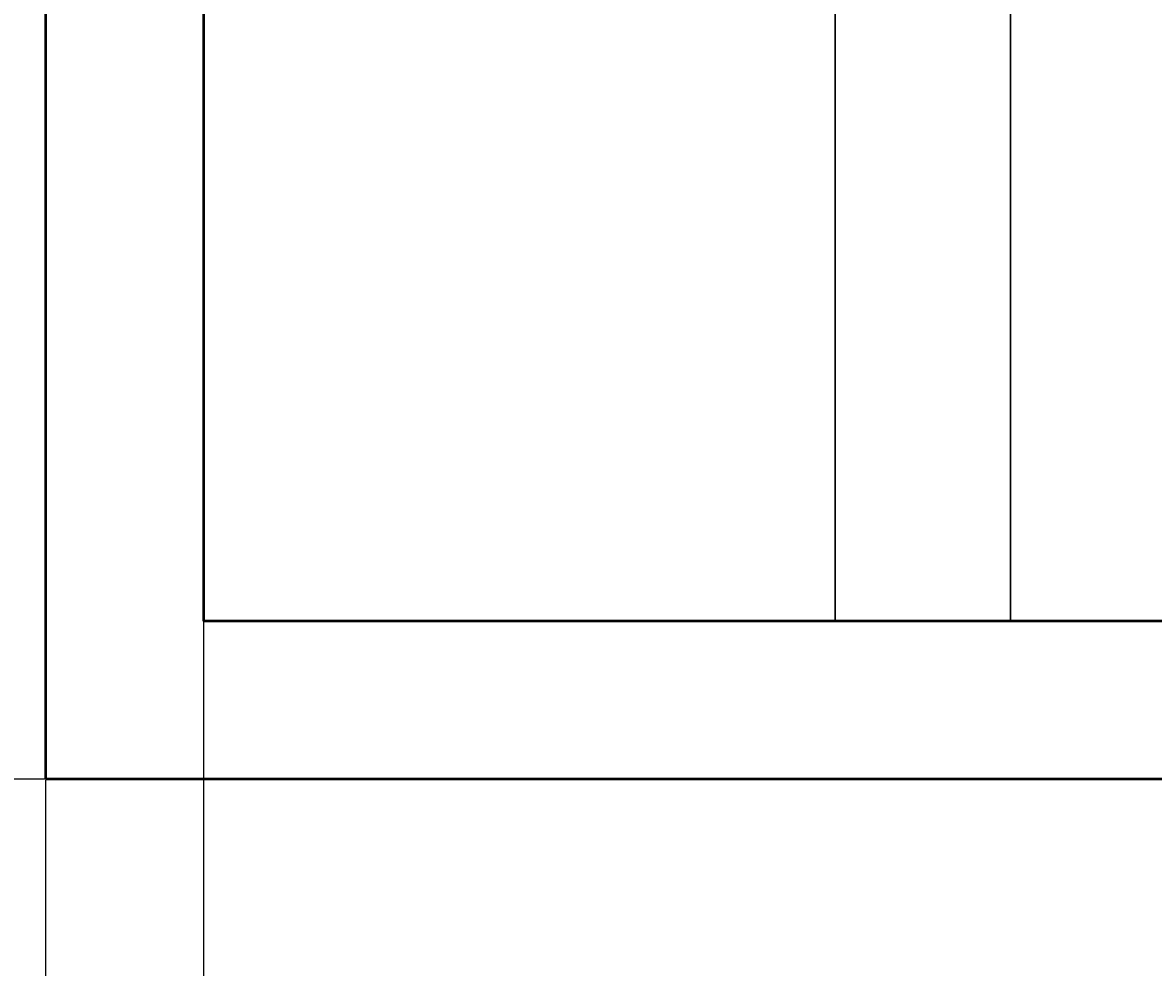
# Model space of a CAD drawing. Units: inches. Extents: x 37 to 824, y -700 to 234.
# Tile 24 of 77: x 160 to 224, y -377 to -323. Entities that reach past the tile are written whole.
import ezdxf

# ---------------------------------------------------------------- set-up
doc = ezdxf.new("R2010")
doc.units = ezdxf.units.IN
doc.header["$MEASUREMENT"] = 0
for name, color, linetype, lineweight in [('A-ANNO-DIMS', 2, 'Continuous', 18), ('A-FLOR-STRS', 1, 'Continuous', 25), ('A-WALL', 2, 'Continuous', 50)]:
    doc.layers.add(name, color=color, linetype=linetype, lineweight=lineweight)
doc.styles.get("Standard").update_dxf_attribs({"font": 'arial.ttf'})
doc.dimstyles.get("Standard").update_dxf_attribs({"dimtxt": 0.18, "dimasz": 0.18, "dimexe": 0.18, "dimexo": 0.0625, "dimgap": 0.09, "dimtad": 0, "dimtih": 1, "dimtoh": 1, "dimdec": 1, "dimzin": 0, "dimdsep": 46, "dimlunit": 4, "dimtxsty": 'Standard', "dimcen": 0.09, "dimadec": 0, "dimazin": 0, "dimtfac": 1, "dimtdec": 1, "dimtofl": 0, "dimtmove": 0, "dimatfit": 3, "dimfxl": 1, "dimtolj": 1, "dimtzin": 0, "dimarcsym": 0})

# ---------------------------------------------------------------- blocks, each defined once
blk = doc.blocks.new('*D59')
at = {"layer": 'A-ANNO-DIMS', "color": 0, "lineweight": -2, "ltscale": 0.5, "transparency": 16777216}
for p, q in [((161.015, -236.91), (78.159, -236.91)), ((78.339, -237.09), (78.339, -301.228)), ((78.339, -365.73), (78.339, -301.591)), ((161.015, -365.91), (78.159, -365.91))]:
    blk.add_line(p, q, dxfattribs=at)
at = {"layer": 'A-ANNO-DIMS', "color": 0, "ltscale": 0.5, "transparency": 16777216}
for points in [[(78.309, -237.09), (78.369, -237.09), (78.339, -236.91)], [(78.309, -365.73), (78.369, -365.73), (78.339, -365.91)]]:
    blk.add_solid(points, dxfattribs=at)
at = {"layer": 'Defpoints', "color": 0, "ltscale": 0.5, "transparency": 16777216}
for p in [(161.077, -236.91), (78.339, -365.91), (161.077, -365.91)]:
    blk.add_point(p, dxfattribs=at)
at = {"layer": 'A-ANNO-DIMS', "color": 0, "ltscale": 0.5, "transparency": 16777216, "insert": (78.339, -301.41), "char_height": 0.18, "attachment_point": 5}
blk.add_mtext('\\A1;10\'-9"', dxfattribs=at)
blk = doc.blocks.new('*D80')
at = {"layer": 'A-ANNO-DIMS', "color": 0, "lineweight": -2, "ltscale": 0.5, "transparency": 16777216}
for p, q in [((170.077, -167.972), (170.077, -400.406)), ((250.19, -167.972), (250.19, -400.406)), ((170.257, -400.226), (209.804, -400.226)), ((250.01, -400.226), (210.463, -400.226))]:
    blk.add_line(p, q, dxfattribs=at)
at = {"layer": 'A-ANNO-DIMS', "color": 0, "ltscale": 0.5, "transparency": 16777216}
for points in [[(170.257, -400.196), (170.257, -400.256), (170.077, -400.226)], [(250.01, -400.196), (250.01, -400.256), (250.19, -400.226)]]:
    blk.add_solid(points, dxfattribs=at)
at = {"layer": 'Defpoints', "color": 0, "ltscale": 0.5, "transparency": 16777216}
for p in [(170.077, -167.91), (250.19, -167.91), (250.19, -400.226)]:
    blk.add_point(p, dxfattribs=at)
at = {"layer": 'A-ANNO-DIMS', "color": 0, "ltscale": 0.5, "transparency": 16777216, "insert": (210.133, -400.226), "char_height": 0.18, "attachment_point": 5}
blk.add_mtext('\\A1;6\'-8"', dxfattribs=at)
blk = doc.blocks.new('*D85')
at = {"layer": 'A-ANNO-DIMS', "color": 0, "lineweight": -2, "ltscale": 0.5, "transparency": 16777216}
for p, q in [((170.077, -356.847), (170.077, 234.17)), ((170.257, 233.99), (187.748, 233.99)), ((205.897, 233.99), (188.406, 233.99)), ((206.077, -356.847), (206.077, 234.17))]:
    blk.add_line(p, q, dxfattribs=at)
at = {"layer": 'A-ANNO-DIMS', "color": 0, "ltscale": 0.5, "transparency": 16777216}
for points in [[(170.257, 234.02), (170.257, 233.96), (170.077, 233.99)], [(205.897, 234.02), (205.897, 233.96), (206.077, 233.99)]]:
    blk.add_solid(points, dxfattribs=at)
at = {"layer": 'Defpoints', "color": 0, "ltscale": 0.5, "transparency": 16777216}
for p in [(206.077, 233.99), (170.077, -356.91), (206.077, -356.91)]:
    blk.add_point(p, dxfattribs=at)
at = {"layer": 'A-ANNO-DIMS', "color": 0, "ltscale": 0.5, "transparency": 16777216, "insert": (188.077, 233.99), "char_height": 0.18, "attachment_point": 5}
blk.add_mtext('\\A1;3\'-0"', dxfattribs=at)
blk = doc.blocks.new('*D86')
at = {"layer": 'A-ANNO-DIMS', "color": 0, "lineweight": -2, "ltscale": 0.5, "transparency": 16777216}
for p, q in [((206.077, -356.847), (206.077, 234.17)), ((206.257, 233.99), (210.678, 233.99)), ((215.897, 233.99), (211.476, 233.99)), ((216.077, -356.847), (216.077, 234.17))]:
    blk.add_line(p, q, dxfattribs=at)
at = {"layer": 'A-ANNO-DIMS', "color": 0, "ltscale": 0.5, "transparency": 16777216}
for points in [[(206.257, 234.02), (206.257, 233.96), (206.077, 233.99)], [(215.897, 234.02), (215.897, 233.96), (216.077, 233.99)]]:
    blk.add_solid(points, dxfattribs=at)
at = {"layer": 'Defpoints', "color": 0, "ltscale": 0.5, "transparency": 16777216}
for p in [(216.077, 233.99), (206.077, -356.91), (216.077, -356.91)]:
    blk.add_point(p, dxfattribs=at)
at = {"layer": 'A-ANNO-DIMS', "color": 0, "ltscale": 0.5, "transparency": 16777216, "insert": (211.077, 233.99), "char_height": 0.18, "attachment_point": 5}
blk.add_mtext('\\A1;0\'-10"', dxfattribs=at)
blk = doc.blocks.new('*D87')
at = {"layer": 'A-ANNO-DIMS', "color": 0, "lineweight": -2, "ltscale": 0.5, "transparency": 16777216}
for p, q in [((216.077, -356.847), (216.077, 234.17)), ((216.257, 233.99), (255.747, 233.99)), ((295.897, 233.99), (256.407, 233.99)), ((296.077, -356.847), (296.077, 234.17))]:
    blk.add_line(p, q, dxfattribs=at)
at = {"layer": 'A-ANNO-DIMS', "color": 0, "ltscale": 0.5, "transparency": 16777216}
for points in [[(216.257, 234.02), (216.257, 233.96), (216.077, 233.99)], [(295.897, 234.02), (295.897, 233.96), (296.077, 233.99)]]:
    blk.add_solid(points, dxfattribs=at)
at = {"layer": 'Defpoints', "color": 0, "ltscale": 0.5, "transparency": 16777216}
for p in [(296.077, 233.99), (216.077, -356.91), (296.077, -356.91)]:
    blk.add_point(p, dxfattribs=at)
at = {"layer": 'A-ANNO-DIMS', "color": 0, "ltscale": 0.5, "transparency": 16777216, "insert": (256.077, 233.99), "char_height": 0.18, "attachment_point": 5}
blk.add_mtext('\\A1;6\'-8"', dxfattribs=at)
blk = doc.blocks.new('*D89')
at = {"layer": 'A-ANNO-DIMS', "color": 0, "lineweight": -2, "ltscale": 0.5, "transparency": 16777216}
for p, q in [((170.077, -356.972), (170.077, -400.406)), ((161.077, -365.972), (161.077, -400.406)), ((161.257, -400.226), (165.248, -400.226)), ((169.897, -400.226), (165.906, -400.226))]:
    blk.add_line(p, q, dxfattribs=at)
at = {"layer": 'A-ANNO-DIMS', "color": 0, "ltscale": 0.5, "transparency": 16777216}
for points in [[(161.257, -400.196), (161.257, -400.256), (161.077, -400.226)], [(169.897, -400.196), (169.897, -400.256), (170.077, -400.226)]]:
    blk.add_solid(points, dxfattribs=at)
at = {"layer": 'Defpoints', "color": 0, "ltscale": 0.5, "transparency": 16777216}
for p in [(170.077, -356.91), (161.077, -365.91), (170.077, -400.226)]:
    blk.add_point(p, dxfattribs=at)
at = {"layer": 'A-ANNO-DIMS', "color": 0, "ltscale": 0.5, "transparency": 16777216, "insert": (165.577, -400.226), "char_height": 0.18, "attachment_point": 5}
blk.add_mtext('\\A1;0\'-9"', dxfattribs=at)

msp = doc.modelspace()

# ---------------------------------------------------------------- linework, layer by layer
at = {"layer": 'A-FLOR-STRS'}
for p, q in [((206.077, -315.91), (206.077, -356.91)), ((216.077, -315.91), (216.077, -356.91))]:
    msp.add_line(p, q, dxfattribs=at)
at = {"layer": 'A-WALL'}
for p, q in [((161.077, 75.09), (161.077, -365.91)), ((170.077, -274.91), (170.077, -356.91)), ((299.077, -356.91), (170.077, -356.91)), ((428.077, -365.91), (161.077, -365.91))]:
    msp.add_line(p, q, dxfattribs=at)

# ---------------------------------------------------------------- dimensions: what is measured, and where the dimension line sits
at = {"layer": 'A-ANNO-DIMS', "ltscale": 0.5}
for base, p1, p2, picture, middle in [((206.077, 233.99), (170.077, -356.91), (206.077, -356.91), '*D85', (188.077, 233.99)), ((216.077, 233.99), (206.077, -356.91), (216.077, -356.91), '*D86', (211.077, 233.99)), ((296.077, 233.99), (216.077, -356.91), (296.077, -356.91), '*D87', (256.077, 233.99)), ((250.19, -400.226), (170.077, -167.91), (250.19, -167.91), '*D80', (210.133, -400.226)), ((170.077, -400.226), (161.077, -365.91), (170.077, -356.91), '*D89', (165.577, -400.226))]:
    dim = msp.add_linear_dim(base=base, p1=p1, p2=p2, dimstyle='Standard', override={"dimdec": 1, "dimlfac": 1, "dimrnd": 0, "dimzin": 1, "dimdsep": 46, "dimlunit": 4, "dimfrac": 2}, dxfattribs=at)
    dim.commit()
    dim.dimension.update_dxf_attribs({"geometry": picture, "text_midpoint": middle})
dim = msp.add_linear_dim(base=(78.339, -365.91), p1=(161.077, -236.91), p2=(161.077, -365.91), angle=90, dimstyle='Standard', override={"dimdec": 1, "dimlfac": 1, "dimrnd": 0, "dimzin": 1, "dimdsep": 46, "dimlunit": 4, "dimfrac": 2}, dxfattribs=at)
dim.commit()
dim.dimension.update_dxf_attribs({"geometry": '*D59', "text_midpoint": (78.339, -301.41)})

doc.saveas('drawing.dxf')
